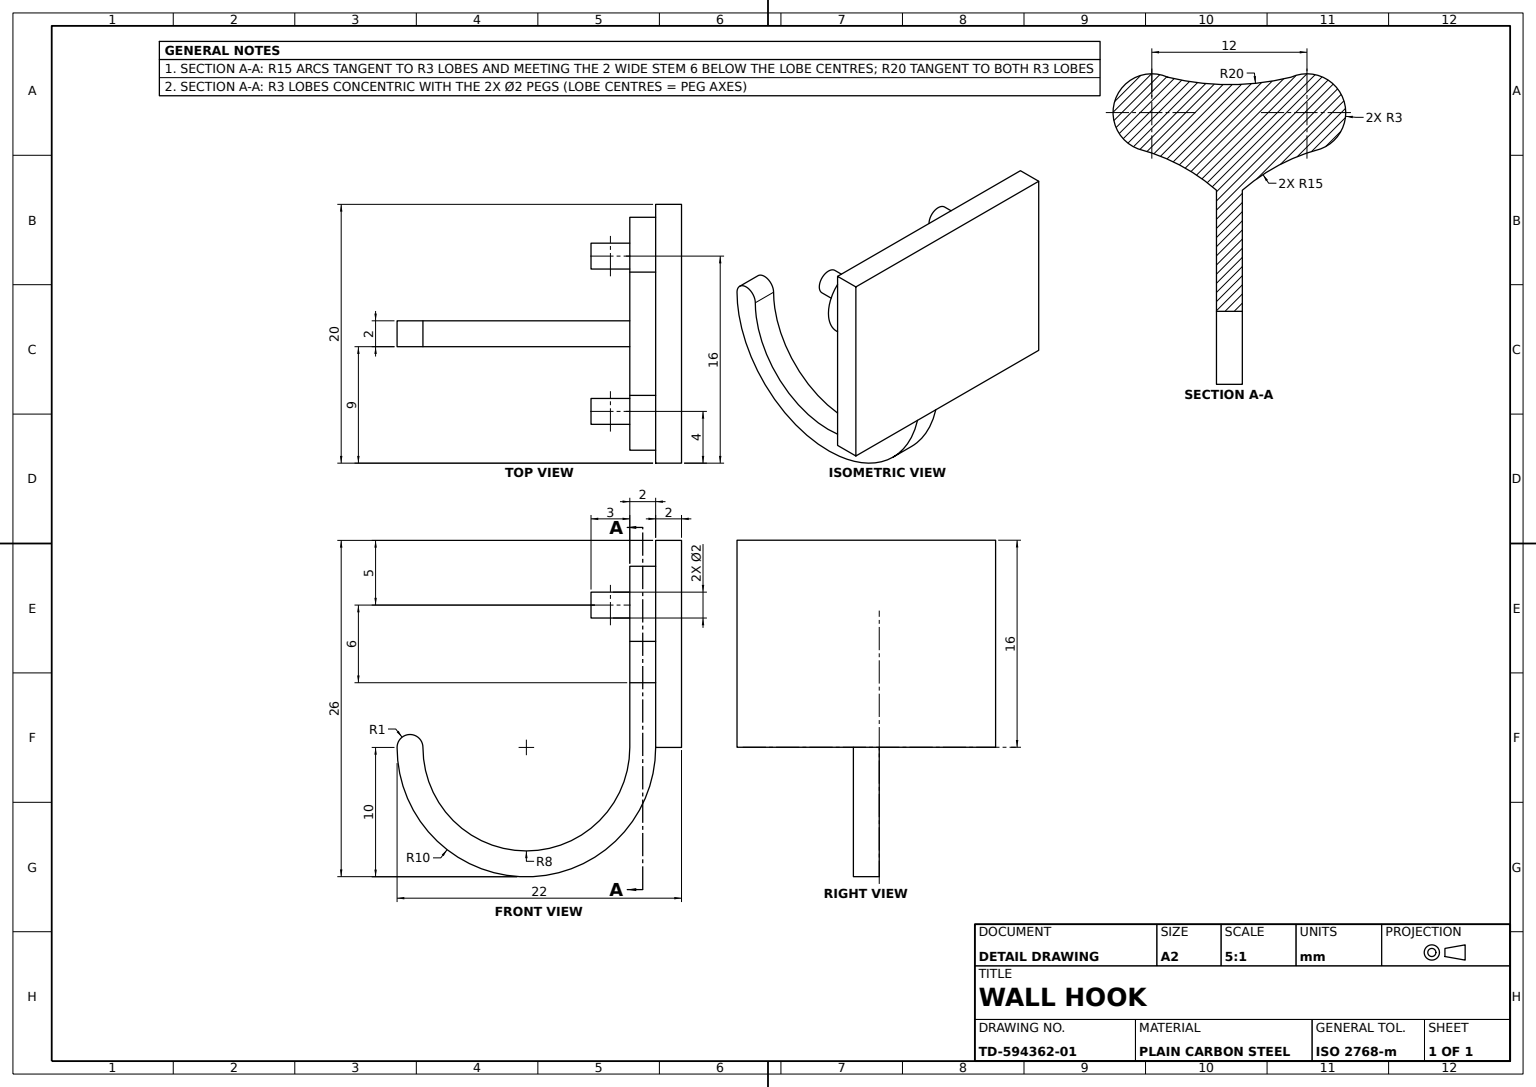
from build123d import *

# Parameters (mm, degrees)
BACK_PLATE_SKETCH_W      = 20
BACK_PLATE_SKETCH_H      = 16
BACK_PLATE_16X20X2_DEPTH = 2
BRACKET_PROFILE_SKETCH_R = 1
HOOK_BRACKET_DEPTH       = 2
PIN_CIRCLES_SKETCH_R     = 1
MOUNTING_PINS_2X_DEPTH   = 5
HOOK_SECTION_SKETCH_W    = 2
HOOK_SECTION_SKETCH_H    = 2
HOOK_TIP_DEPTH           = 2


with BuildPart() as part:
    # Back Plate Sketch → Back Plate 16x20x2 (new body)
    with BuildSketch(Plane.XY):
        Rectangle(BACK_PLATE_SKETCH_W, BACK_PLATE_SKETCH_H)
    extrude(amount=BACK_PLATE_16X20X2_DEPTH)

    # Bracket Profile Sketch → Hook Bracket (add)
    with BuildSketch(Plane.XY.offset(2)):
        with BuildLine():
            Line((-1, -3), (-1, -8))
            Line((-1, -8), (1, -8))
            Line((1, -8), (1, -3))
            ThreePointArc((1, -3), (3.84680434, -1.051653316), (7.06343132, 0.19480592))
            ThreePointArc((7.06343132, 0.19480592), (8.770582601, 4.150596389), (4.76336302, 5.73326343))
            ThreePointArc((4.76336302, 5.73326343), (0, 5.15774213), (-4.76336302, 5.73326343))
            ThreePointArc((-4.76336302, 5.73326343), (-8.770582601, 4.150596389), (-7.06343132, 0.19480592))
            ThreePointArc((-7.06343132, 0.19480592), (-3.84680434, -1.051653316), (-1, -3))
        make_face()
        with Locations((-6, 3)):
            Circle(BRACKET_PROFILE_SKETCH_R, mode=Mode.SUBTRACT)
        with Locations(Location((6, 3, 0), (0, 0, 180))):
            Circle(BRACKET_PROFILE_SKETCH_R, mode=Mode.SUBTRACT)
    extrude(amount=HOOK_BRACKET_DEPTH)

    # Pin Circles Sketch → Mounting Pins 2x (add)
    with BuildSketch(Plane.XY.offset(2)):
        with Locations((-6, 3)):
            Circle(PIN_CIRCLES_SKETCH_R)
        with Locations(Location((6, 3, 0), (0, 0, 180))):
            Circle(PIN_CIRCLES_SKETCH_R)
    extrude(amount=MOUNTING_PINS_2X_DEPTH)

    # Hook Arm Sweep: sweep along a path in Hook Path Sketch
    with BuildLine(Plane(origin=(0, 0, 0), x_dir=(0, 0, -1), z_dir=(1, 0, 0))) as hook_arm_sweep_path:
        ThreePointArc((-3, -8), (-12, -17), (-21, -8))
    # Hook Section Sketch → Hook Arm Sweep (sweep)
    with BuildSketch(Plane.XZ.offset(8)):
        with Locations((0, 3)):
            Rectangle(HOOK_SECTION_SKETCH_W, HOOK_SECTION_SKETCH_H)
    sweep(path=hook_arm_sweep_path.line)

    # Hook Tip Sketch → Hook Tip (add)
    with BuildSketch(Plane.ZY.offset(1)):
        with BuildLine():
            Line((20, -8), (22, -8))
            ThreePointArc((22, -8), (21, -7), (20, -8))
        make_face()
    extrude(amount=-HOOK_TIP_DEPTH)


solid = part.part
